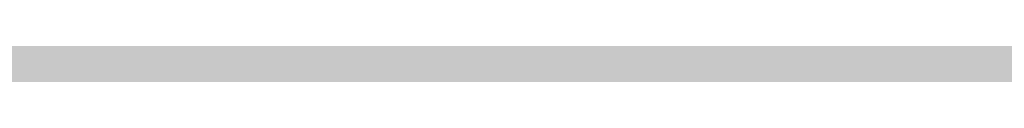
# Model space of a CAD drawing. Units: millimetres. Extents: x 0 to 2267, y 0 to 1823.
# Tile 55 of 256: x 1596.855 to 1600.369, y 1227.171 to 1227.246. Entities that reach past the tile are written whole.
import ezdxf

# ---------------------------------------------------------------- set-up
doc = ezdxf.new("R2010")
doc.units = ezdxf.units.MM
doc.header["$MEASUREMENT"] = 0
doc.layers.add('M-HATC', color=252, linetype='Continuous', lineweight=18)

msp = doc.modelspace()

# ---------------------------------------------------------------- hatches: boundary and pattern name
at = {"layer": 'M-HATC'}
h = msp.add_hatch(color=256, dxfattribs=at)
h.dxf.hatch_style = 1
h.paths.add_polyline_path([(2055.771, 1603.062), (1381.0868, 1603.062), (1381.0868, 1598.062), (2055.771, 1598.062)])
h.paths.add_polyline_path([(2055.771, 1598.062), (1381.0868, 1598.062), (1381.0868, 1593.062), (2055.771, 1593.062)])
h.paths.add_polyline_path([(2051.3074, 1536.7609), (1385.5504, 1536.7609), (1385.5504, 1526.7609), (1387.5504, 1526.7609), (1388.5366, 1525.0528), (1385.3319, 1521.2335), (1385.3319, 1521.2226), (2050.2542, 1522.7491), (2048.3212, 1525.0528), (2049.3074, 1526.7609), (2051.3074, 1526.7609)])
edge = h.paths.add_edge_path()
edge.add_arc((1847.5345, 1379.1492), 135, 222.603061, 222.890851, ccw=False)
edge.add_line((1748.1663, 1287.7656), (1683.0921, 1287.7656))
edge.add_arc((1583.7239, 1379.1492), 135, 317.109149, 317.396939, ccw=False)
edge.add_arc((1678.9686, 1290.6707), 5, 222.8909, 317.1091, ccw=False)
edge.add_arc((1774.2133, 1379.1492), 135, 222.603061, 222.890851, ccw=False)
edge.add_line((1674.8451, 1287.7656), (1609.7709, 1287.7656))
edge.add_arc((1510.4027, 1379.1492), 135, 317.109149, 317.396939, ccw=False)
edge.add_arc((1605.6474, 1290.6707), 5, 222.8909, 317.1091, ccw=False)
edge.add_arc((1700.8921, 1379.1492), 135, 222.603061, 222.890851, ccw=False)
edge.add_line((1601.5239, 1287.7656), (1536.4497, 1287.7656))
edge.add_arc((1437.0815, 1379.1492), 135, 317.109149, 317.396939, ccw=False)
edge.add_arc((1532.3262, 1290.6707), 5, 222.8909, 317.1091, ccw=False)
edge.add_arc((1627.5709, 1379.1492), 135, 222.603061, 222.890851, ccw=False)
edge.add_line((1528.2027, 1287.7656), (1505.9289, 1287.7656))
edge.add_spline(control_points=[(1505.9289, 1287.7656), (1504.2622, 1287.7656), (1504.2622, 1282.7656), (1505.9289, 1282.7656)], knot_values=[0, 0, 0, 0, 5, 5, 5, 5], degree=3, periodic=0)
edge.add_line((1505.9289, 1282.7656), (1930.9289, 1282.7656))
edge.add_spline(control_points=[(1930.9289, 1282.7656), (1932.5956, 1282.7656), (1932.5956, 1287.7656), (1930.9289, 1287.7656)], knot_values=[0, 0, 0, 0, 5, 5, 5, 5], degree=3, periodic=0)
edge.add_line((1930.9289, 1287.7656), (1903.0557, 1287.7656))
edge.add_arc((1803.6875, 1379.1492), 135, 317.109149, 317.396939, ccw=False)
edge.add_arc((1898.9322, 1290.6707), 5, 222.8909, 317.1091, ccw=False)
edge.add_arc((1994.1769, 1379.1492), 135, 222.603061, 222.890851, ccw=False)
edge.add_line((1894.8087, 1287.7656), (1829.7345, 1287.7656))
edge.add_arc((1730.3663, 1379.1492), 135, 317.109149, 317.396939, ccw=False)
edge.add_arc((1825.611, 1290.6707), 5, 222.8909, 317.1091, ccw=False)
edge.add_arc((1920.8557, 1379.1492), 135, 222.603061, 222.890851, ccw=False)
edge.add_line((1821.4875, 1287.7656), (1756.4133, 1287.7656))
edge.add_arc((1657.0451, 1379.1492), 135, 317.109149, 317.396939, ccw=False)
edge.add_arc((1752.2898, 1290.6707), 5, 222.8909, 317.1091, ccw=False)
edge = h.paths.add_edge_path()
edge.add_spline(control_points=[(1843.4289, 1227.2475), (1845.0956, 1227.2475), (1845.0956, 1232.2475), (1843.4289, 1232.2475)], knot_values=[0, 0, 0, 0, 5, 5, 5, 5], degree=3, periodic=0)
edge.add_line((1843.4289, 1232.2475), (1593.4289, 1232.2475))
edge.add_spline(control_points=[(1593.4289, 1232.2475), (1591.7622, 1232.2475), (1591.7622, 1227.2475), (1593.4289, 1227.2475)], knot_values=[0, 0, 0, 0, 5, 5, 5, 5], degree=3, periodic=0)
edge.add_line((1593.4289, 1227.2475), (1843.4289, 1227.2475))
h.paths.add_polyline_path([(1905.9289, 1127.4171), (1530.9289, 1127.4171, 0.414214), (1520.9289, 1117.4171), (1530.9289, 1117.4171), (1915.9289, 1117.4171, 0.414214)])
edge = h.paths.add_edge_path()
edge.add_arc((1397.0858, 1498.4078), 12.7299, 90.78215, 190.87871, ccw=False)
edge.add_line((1396.912, 1511.1365), (1428.0097, 1511.3488))
edge.add_line((1428.0097, 1511.3488), (1433.0097, 1511.3488))
edge.add_line((1433.0097, 1511.3488), (1434.439, 1511.3488))
edge.add_arc((1419.474, 1498.0804), 20, 41.561, 74.08211)
edge.add_line((1424.9592, 1517.3135), (1399.9351, 1517.2561))
edge.add_spline(control_points=[(1399.9307, 1517.2561), (1399.884, 1517.2131), (1399.8328, 1517.1689), (1399.7774, 1517.1236)], knot_values=[11.567499, 11.567499, 11.567499, 11.567499, 11.814249, 11.814249, 11.814249, 11.814249], degree=3, periodic=0)
edge.add_spline(control_points=[(1399.6328, 1517.0099), (1399.5831, 1516.9721), (1399.5307, 1516.9338), (1399.4759, 1516.8947)], knot_values=[11.167718, 11.167718, 11.167718, 11.167718, 11.365188, 11.365188, 11.365188, 11.365188], degree=3, periodic=0)
edge.add_spline(control_points=[(1399.3398, 1516.8001), (1399.1514, 1516.6719), (1398.9384, 1516.5377), (1398.704, 1516.3994)], knot_values=[10.376405, 10.376405, 10.376405, 10.376405, 11.00994, 11.00994, 11.00994, 11.00994], degree=3, periodic=0)
edge.add_spline(control_points=[(1398.6572, 1516.3719), (1398.5789, 1516.326), (1398.4983, 1516.2797), (1398.4155, 1516.2331)], knot_values=[10.125175, 10.125175, 10.125175, 10.125175, 10.334406, 10.334406, 10.334406, 10.334406], degree=3, periodic=0)
edge.add_spline(control_points=[(1398.2642, 1516.1487), (1398.196, 1516.1111), (1398.1263, 1516.0732), (1398.0555, 1516.0351)], knot_values=[9.832246, 9.832246, 9.832246, 9.832246, 9.999658, 9.999658, 9.999658, 9.999658], degree=3, periodic=0)
edge.add_spline(control_points=[(1397.9987, 1516.0048), (1397.7312, 1515.8621), (1397.446, 1515.7171), (1397.1466, 1515.5714)], knot_values=[9.161808, 9.161808, 9.161808, 9.161808, 9.787769, 9.787769, 9.787769, 9.787769], degree=3, periodic=0)
edge.add_spline(control_points=[(1397.1466, 1515.5714), (1396.8418, 1515.423), (1396.5222, 1515.274), (1396.1914, 1515.1262)], knot_values=[8.524455, 8.524455, 8.524455, 8.524455, 9.161808, 9.161808, 9.161808, 9.161808], degree=3, periodic=0)
edge.add_spline(control_points=[(1396.0777, 1515.0756), (1395.9854, 1515.0348), (1395.8922, 1514.994), (1395.7983, 1514.9534)], knot_values=[8.275193, 8.275193, 8.275193, 8.275193, 8.451726, 8.451726, 8.451726, 8.451726], degree=3, periodic=0)
edge.add_spline(control_points=[(1395.6018, 1514.8691), (1395.4997, 1514.8257), (1395.3968, 1514.7824), (1395.2932, 1514.7394)], knot_values=[7.962917, 7.962917, 7.962917, 7.962917, 8.152764, 8.152764, 8.152764, 8.152764], degree=3, periodic=0)
edge.add_spline(control_points=[(1395.2116, 1514.7057), (1394.8278, 1514.5475), (1394.4345, 1514.3929), (1394.0364, 1514.2442)], knot_values=[7.21254, 7.21254, 7.21254, 7.21254, 7.913148, 7.913148, 7.913148, 7.913148], degree=3, periodic=0)
edge.add_spline(control_points=[(1394.0364, 1514.2442), (1393.7076, 1514.1214), (1393.3754, 1514.0027), (1393.0427, 1513.8895)], knot_values=[6.633733, 6.633733, 6.633733, 6.633733, 7.21254, 7.21254, 7.21254, 7.21254], degree=3, periodic=0)
edge.add_spline(control_points=[(1392.8214, 1513.815), (1392.7198, 1513.7812), (1392.6181, 1513.7479), (1392.5166, 1513.7152)], knot_values=[6.328796, 6.328796, 6.328796, 6.328796, 6.505493, 6.505493, 6.505493, 6.505493], degree=3, periodic=0)
edge.add_spline(control_points=[(1392.5166, 1513.7152), (1392.3187, 1513.6515), (1392.1212, 1513.59), (1391.9244, 1513.531)], knot_values=[5.984605, 5.984605, 5.984605, 5.984605, 6.328796, 6.328796, 6.328796, 6.328796], degree=3, periodic=0)
edge.add_spline(control_points=[(1391.7915, 1513.4915), (1391.3122, 1513.3501), (1390.8384, 1513.2239), (1390.3784, 1513.1171)], knot_values=[5.066697, 5.066697, 5.066697, 5.066697, 5.907055, 5.907055, 5.907055, 5.907055], degree=3, periodic=0)
edge.add_spline(control_points=[(1390.3784, 1513.1171), (1390.1797, 1513.071), (1389.9836, 1513.0284), (1389.7907, 1512.9899)], knot_values=[4.70367, 4.70367, 4.70367, 4.70367, 5.066695, 5.066695, 5.066695, 5.066695], degree=3, periodic=0)
edge.add_spline(control_points=[(1389.422, 1512.9204), (1389.2459, 1512.8892), (1389.0729, 1512.8617), (1388.9036, 1512.8381)], knot_values=[4.130571, 4.130571, 4.130571, 4.130571, 4.469816, 4.469816, 4.469816, 4.469816], degree=3, periodic=0)
edge.add_spline(control_points=[(1388.9036, 1512.8381), (1388.591, 1512.7946), (1388.2911, 1512.7644), (1388.0071, 1512.7494)], knot_values=[3.504031, 3.504031, 3.504031, 3.504031, 4.130571, 4.130571, 4.130571, 4.130571], degree=3, periodic=0)
edge.add_spline(control_points=[(1387.9356, 1512.7459), (1387.8538, 1512.7423), (1387.7733, 1512.74), (1387.6944, 1512.739)], knot_values=[3.268866, 3.268866, 3.268866, 3.268866, 3.451164, 3.451164, 3.451164, 3.451164], degree=3, periodic=0)
edge.add_spline(control_points=[(1387.3351, 1512.7443), (1387.2076, 1512.7499), (1387.0847, 1512.7597), (1386.967, 1512.7739)], knot_values=[2.670686, 2.670686, 2.670686, 2.670686, 2.984, 2.984, 2.984, 2.984], degree=3, periodic=0)
edge.add_spline(control_points=[(1386.8327, 1512.7922), (1386.8209, 1512.7941), (1386.8092, 1512.7959), (1386.7975, 1512.7979)], knot_values=[2.516981, 2.516981, 2.516981, 2.516981, 2.549528, 2.549528, 2.549528, 2.549528], degree=3, periodic=0)
edge.add_spline(control_points=[(1386.4526, 1512.8735), (1386.4257, 1512.881), (1386.3993, 1512.889), (1386.3733, 1512.8972)], knot_values=[2.095869, 2.095869, 2.095869, 2.095869, 2.17941, 2.17941, 2.17941, 2.17941], degree=3, periodic=0)
edge.add_spline(control_points=[(1386.0691, 1513.0189), (1386.0634, 1513.0217), (1386.0577, 1513.0246), (1386.052, 1513.0275)], knot_values=[1.72453, 1.72453, 1.72453, 1.72453, 1.745933, 1.745933, 1.745933, 1.745933], degree=3, periodic=0)
edge.add_arc((1399.474, 1498.0804), 20, 131.82432, 180)
edge.add_arc((1630.3336, 1505.5484), 250.9708, 181.705176, 236.427975)
edge.add_arc((1605.3399, 1483.3044), 218.7822, 238.660829, 243.34961)
edge.add_arc((1647.0911, 1510.3592), 262.8986, 183.129836, 237.853442, ccw=False)
h.paths.add_polyline_path([(1406.5369, 1391.9644, 0.149382), (1491.5506, 1296.4418, -0.129517)], flags=17)
edge = h.paths.add_edge_path()
edge.add_arc((2037.3838, 1498.0804), 20, 0, 48.26587)
edge.add_spline(control_points=[(2050.6973, 1513.0052), (2050.6512, 1512.9847), (2050.6034, 1512.9655), (2050.5539, 1512.9477)], knot_values=[1.835652, 1.835652, 1.835652, 1.835652, 2.000781, 2.000781, 2.000781, 2.000781], degree=3, periodic=0)
edge.add_spline(control_points=[(2050.4616, 1512.9166), (2050.479, 1512.9221), (2050.4963, 1512.9277), (2050.5133, 1512.9335)], knot_values=[2.045477, 2.045477, 2.045477, 2.045477, 2.101389, 2.101389, 2.101389, 2.101389], degree=3, periodic=0)
edge.add_spline(control_points=[(2050.129, 1512.8342), (2050.1984, 1512.8473), (2050.2657, 1512.8623), (2050.3308, 1512.8792)], knot_values=[2.237629, 2.237629, 2.237629, 2.237629, 2.435841, 2.435841, 2.435841, 2.435841], degree=3, periodic=0)
edge.add_spline(control_points=[(2050.0946, 1512.8278), (2050.1061, 1512.8299), (2050.1176, 1512.832), (2050.129, 1512.8342)], knot_values=[2.435841, 2.435841, 2.435841, 2.435841, 2.468321, 2.468321, 2.468321, 2.468321], degree=3, periodic=0)
edge.add_spline(control_points=[(2049.7843, 1512.7851), (2049.8552, 1512.7922), (2049.9243, 1512.8008), (2049.9917, 1512.8109)], knot_values=[2.563852, 2.563852, 2.563852, 2.563852, 2.748541, 2.748541, 2.748541, 2.748541], degree=3, periodic=0)
edge.add_spline(control_points=[(2049.4052, 1512.7617), (2049.5364, 1512.7653), (2049.6629, 1512.773), (2049.7843, 1512.7851)], knot_values=[2.748541, 2.748541, 2.748541, 2.748541, 3.064882, 3.064882, 3.064882, 3.064882], degree=3, periodic=0)
edge.add_spline(control_points=[(2049.1698, 1512.7597), (2049.2336, 1512.7591), (2049.2965, 1512.7594), (2049.3584, 1512.7606)], knot_values=[3.102309, 3.102309, 3.102309, 3.102309, 3.2503, 3.2503, 3.2503, 3.2503], degree=3, periodic=0)
edge.add_spline(control_points=[(2048.8573, 1512.7691), (2048.9638, 1512.7638), (2049.068, 1512.7606), (2049.1698, 1512.7597)], knot_values=[3.2503, 3.2503, 3.2503, 3.2503, 3.486069, 3.486069, 3.486069, 3.486069], degree=3, periodic=0)
edge.add_spline(control_points=[(2048.6924, 1512.7789), (2048.3729, 1512.8009), (2048.0345, 1512.8411), (2047.6817, 1512.897)], knot_values=[3.606429, 3.606429, 3.606429, 3.606429, 4.2989, 4.2989, 4.2989, 4.2989], degree=3, periodic=0)
edge.add_spline(control_points=[(2047.6817, 1512.897), (2047.5458, 1512.9185), (2047.4077, 1512.9424), (2047.2678, 1512.9685)], knot_values=[4.2989, 4.2989, 4.2989, 4.2989, 4.565769, 4.565769, 4.565769, 4.565769], degree=3, periodic=0)
edge.add_spline(control_points=[(2047.2678, 1512.9685), (2047.1449, 1512.9914), (2047.0207, 1513.016), (2046.8951, 1513.0422)], knot_values=[4.565769, 4.565769, 4.565769, 4.565769, 4.799971, 4.799971, 4.799971, 4.799971], degree=3, periodic=0)
edge.add_spline(control_points=[(2046.8951, 1513.0422), (2046.5286, 1513.1188), (2046.1513, 1513.209), (2045.7676, 1513.3107)], knot_values=[4.799971, 4.799971, 4.799971, 4.799971, 5.483718, 5.483718, 5.483718, 5.483718], degree=3, periodic=0)
edge.add_spline(control_points=[(2045.7676, 1513.3107), (2045.3724, 1513.4154), (2044.9704, 1513.5322), (2044.5662, 1513.6588)], knot_values=[5.483718, 5.483718, 5.483718, 5.483718, 6.187866, 6.187866, 6.187866, 6.187866], degree=3, periodic=0)
edge.add_spline(control_points=[(2044.5662, 1513.6588), (2044.4149, 1513.7061), (2044.2633, 1513.7549), (2044.1116, 1513.8048)], knot_values=[6.187866, 6.187866, 6.187866, 6.187866, 6.451551, 6.451551, 6.451551, 6.451551], degree=3, periodic=0)
edge.add_spline(control_points=[(2044.1116, 1513.8048), (2043.9967, 1513.8427), (2043.8817, 1513.8813), (2043.7668, 1513.9205)], knot_values=[6.451551, 6.451551, 6.451551, 6.451551, 6.651434, 6.651434, 6.651434, 6.651434], degree=3, periodic=0)
edge.add_spline(control_points=[(2043.7668, 1513.9205), (2043.3716, 1514.0554), (2042.9774, 1514.1979), (2042.5886, 1514.3458)], knot_values=[6.651434, 6.651434, 6.651434, 6.651434, 7.338879, 7.338879, 7.338879, 7.338879], degree=3, periodic=0)
edge.add_spline(control_points=[(2042.5886, 1514.3458), (2042.1643, 1514.5071), (2041.7465, 1514.6749), (2041.3409, 1514.846)], knot_values=[7.338879, 7.338879, 7.338879, 7.338879, 8.089209, 8.089209, 8.089209, 8.089209], degree=3, periodic=0)
edge.add_spline(control_points=[(2041.3409, 1514.846), (2041.1028, 1514.9465), (2040.869, 1515.0481), (2040.6405, 1515.1502)], knot_values=[8.089209, 8.089209, 8.089209, 8.089209, 8.529587, 8.529587, 8.529587, 8.529587], degree=3, periodic=0)
edge.add_spline(control_points=[(2040.51, 1515.2089), (2040.0824, 1515.4022), (2039.6747, 1515.5971), (2039.295, 1515.7894)], knot_values=[8.613818, 8.613818, 8.613818, 8.613818, 9.44571, 9.44571, 9.44571, 9.44571], degree=3, periodic=0)
edge.add_spline(control_points=[(2039.295, 1515.7894), (2039.0618, 1515.9075), (2038.8391, 1516.0246), (2038.6288, 1516.1398)], knot_values=[9.44571, 9.44571, 9.44571, 9.44571, 9.956404, 9.956404, 9.956404, 9.956404], degree=3, periodic=0)
edge.add_spline(control_points=[(2038.6288, 1516.1398), (2038.5187, 1516.2001), (2038.4121, 1516.2598), (2038.309, 1516.3189)], knot_values=[9.956404, 9.956404, 9.956404, 9.956404, 10.223542, 10.223542, 10.223542, 10.223542], degree=3, periodic=0)
edge.add_spline(control_points=[(2038.309, 1516.3189), (2038.2138, 1516.3735), (2038.1216, 1516.4276), (2038.0328, 1516.481)], knot_values=[10.223542, 10.223542, 10.223542, 10.223542, 10.47051, 10.47051, 10.47051, 10.47051], degree=3, periodic=0)
edge.add_spline(control_points=[(2038.0328, 1516.481), (2037.7855, 1516.6296), (2037.5639, 1516.773), (2037.3722, 1516.909)], knot_values=[10.47051, 10.47051, 10.47051, 10.47051, 11.15767, 11.15767, 11.15767, 11.15767], degree=3, periodic=0)
edge.add_spline(control_points=[(2037.3722, 1516.909), (2037.2789, 1516.9752), (2037.1927, 1517.0396), (2037.1142, 1517.102)], knot_values=[11.15767, 11.15767, 11.15767, 11.15767, 11.49227, 11.49227, 11.49227, 11.49227], degree=3, periodic=0)
edge.add_spline(control_points=[(2036.8564, 1517.3259), (2036.9148, 1517.2692), (2036.9814, 1517.2103), (2037.0557, 1517.1492)], knot_values=[11.577341, 11.577341, 11.577341, 11.577341, 11.91035, 11.91035, 11.91035, 11.91035], degree=3, periodic=0)
edge.add_spline(control_points=[(2036.8074, 1517.3748), (2036.823, 1517.3587), (2036.8393, 1517.3424), (2036.8564, 1517.3259)], knot_values=[11.91035, 11.91035, 11.91035, 11.91035, 12.007402, 12.007402, 12.007402, 12.007402], degree=3, periodic=0)
edge.add_spline(control_points=[(2036.7017, 1517.494), (2036.7104, 1517.483), (2036.7196, 1517.4719), (2036.7291, 1517.4606)], knot_values=[12.184155, 12.184155, 12.184155, 12.184155, 12.255409, 12.255409, 12.255409, 12.255409], degree=3, periodic=0)
edge.add_spline(control_points=[(2036.6159, 1517.6205), (2036.62, 1517.613), (2036.6243, 1517.6055), (2036.6289, 1517.5979)], knot_values=[12.487913, 12.487913, 12.487913, 12.487913, 12.541035, 12.541035, 12.541035, 12.541035], degree=3, periodic=0)
edge.add_spline(control_points=[(2036.5635, 1517.786), (2036.5637, 1517.7794), (2036.5642, 1517.7726), (2036.565, 1517.7658)], knot_values=[12.911761, 12.911761, 12.911761, 12.911761, 12.968286, 12.968286, 12.968286, 12.968286], degree=3, periodic=0)
edge.add_spline(control_points=[(2036.6166, 1517.9304), (2036.6125, 1517.9259), (2036.6086, 1517.9212), (2036.6049, 1517.9165)], knot_values=[13.382527, 13.382527, 13.382527, 13.382527, 13.433791, 13.433791, 13.433791, 13.433791], degree=3, periodic=0)
edge.add_spline(control_points=[(2036.749, 1518.017), (2036.7361, 1518.0116), (2036.7239, 1518.006), (2036.7124, 1518.0002)], knot_values=[13.726299, 13.726299, 13.726299, 13.726299, 13.809928, 13.809928, 13.809928, 13.809928], degree=3, periodic=0)
edge.add_spline(control_points=[(2036.8604, 1518.0528), (2036.8386, 1518.0474), (2036.8181, 1518.0416), (2036.7988, 1518.0353)], knot_values=[13.910887, 13.910887, 13.910887, 13.910887, 14.02153, 14.02153, 14.02153, 14.02153], degree=3, periodic=0)
edge.add_line((2036.9639, 1518.0804), (2032.3838, 1518.0804))
edge.add_line((2032.3838, 1518.0804), (2027.3838, 1518.0804))
edge.add_line((2027.3838, 1518.0804), (2022.3838, 1518.0804))
edge.add_line((2022.3838, 1518.0804), (2017.3838, 1518.0804))
edge.add_arc((2017.3838, 1498.0804), 20, 90, 138.439)
edge.add_line((2002.4188, 1511.3488), (2003.8481, 1511.3488))
edge.add_line((2003.8481, 1511.3488), (2008.8481, 1511.3488))
edge.add_line((2008.8481, 1511.3488), (2039.772, 1511.1377))
edge.add_arc((2039.772, 1498.4078), 12.7299, -10.87871, 90, ccw=False)
edge.add_arc((1789.7668, 1510.3592), 262.8986, 302.146558, 356.870164, ccw=False)
edge.add_arc((1831.5179, 1483.3044), 218.7822, 296.65039, 301.339171)
edge.add_arc((1806.5242, 1505.5484), 250.9708, 303.572025, 358.294824)
h.paths.add_polyline_path([(2030.321, 1391.9644, -0.129517), (1945.3072, 1296.4418, 0.149382)], flags=17)
edge = h.paths.add_edge_path()
edge.add_spline(control_points=[(2037.2464, 1518.0821), (2037.2898, 1518.081), (2037.3355, 1518.0804), (2037.3838, 1518.0804)], knot_values=[0.000012, 0.000012, 0.000012, 0.000012, 0.144754, 0.144754, 0.144754, 0.144754], degree=3, periodic=0)
edge.add_line((2037.3357, 1518.0804), (2037.0096, 1518.0804))
edge.add_spline(control_points=[(2037.0096, 1518.0804), (2036.9822, 1518.0768), (2036.956, 1518.0727), (2036.9312, 1518.0681)], knot_values=[14.13465, 14.13465, 14.13465, 14.13465, 14.247197, 14.247197, 14.247197, 14.247197], degree=3, periodic=0)
edge.add_spline(control_points=[(2036.9312, 1518.0681), (2036.9276, 1518.0674), (2036.9241, 1518.0667), (2036.9205, 1518.0661)], knot_values=[14.118315, 14.118315, 14.118315, 14.118315, 14.13465, 14.13465, 14.13465, 14.13465], degree=3, periodic=0)
edge.add_spline(control_points=[(2036.9205, 1518.0661), (2036.9118, 1518.0644), (2036.9032, 1518.0626), (2036.8948, 1518.0608)], knot_values=[14.078086, 14.078086, 14.078086, 14.078086, 14.118315, 14.118315, 14.118315, 14.118315], degree=3, periodic=0)
edge.add_spline(control_points=[(2036.8948, 1518.0608), (2036.883, 1518.0583), (2036.8716, 1518.0556), (2036.8604, 1518.0528)], knot_values=[14.02153, 14.02153, 14.02153, 14.02153, 14.078086, 14.078086, 14.078086, 14.078086], degree=3, periodic=0)
edge.add_spline(control_points=[(2036.8604, 1518.0528), (2036.8386, 1518.0474), (2036.8181, 1518.0416), (2036.7988, 1518.0353)], knot_values=[13.910887, 13.910887, 13.910887, 13.910887, 14.02153, 14.02153, 14.02153, 14.02153], degree=3, periodic=0)
edge.add_spline(control_points=[(2036.7988, 1518.0353), (2036.7981, 1518.035), (2036.7974, 1518.0348), (2036.7967, 1518.0346)], knot_values=[13.906906, 13.906906, 13.906906, 13.906906, 13.910887, 13.910887, 13.910887, 13.910887], degree=3, periodic=0)
edge.add_spline(control_points=[(2036.7967, 1518.0346), (2036.7882, 1518.0318), (2036.7799, 1518.0289), (2036.7719, 1518.0259)], knot_values=[13.857826, 13.857826, 13.857826, 13.857826, 13.906906, 13.906906, 13.906906, 13.906906], degree=3, periodic=0)
edge.add_spline(control_points=[(2036.7719, 1518.0259), (2036.764, 1518.023), (2036.7564, 1518.02), (2036.749, 1518.017)], knot_values=[13.809928, 13.809928, 13.809928, 13.809928, 13.857826, 13.857826, 13.857826, 13.857826], degree=3, periodic=0)
edge.add_spline(control_points=[(2036.749, 1518.017), (2036.7361, 1518.0116), (2036.7239, 1518.006), (2036.7124, 1518.0002)], knot_values=[13.726299, 13.726299, 13.726299, 13.726299, 13.809928, 13.809928, 13.809928, 13.809928], degree=3, periodic=0)
edge.add_spline(control_points=[(2036.7124, 1518.0002), (2036.7121, 1518), (2036.7118, 1517.9999), (2036.7115, 1517.9997)], knot_values=[13.723993, 13.723993, 13.723993, 13.723993, 13.726299, 13.726299, 13.726299, 13.726299], degree=3, periodic=0)
edge.add_spline(control_points=[(2036.7115, 1517.9997), (2036.7063, 1517.9971), (2036.7013, 1517.9944), (2036.6965, 1517.9917)], knot_values=[13.686536, 13.686536, 13.686536, 13.686536, 13.723993, 13.723993, 13.723993, 13.723993], degree=3, periodic=0)
edge.add_spline(control_points=[(2036.6965, 1517.9917), (2036.6919, 1517.9891), (2036.6874, 1517.9865), (2036.6831, 1517.9839)], knot_values=[13.651251, 13.651251, 13.651251, 13.651251, 13.686536, 13.686536, 13.686536, 13.686536], degree=3, periodic=0)
edge.add_spline(control_points=[(2036.6831, 1517.9839), (2036.6764, 1517.9798), (2036.67, 1517.9757), (2036.6639, 1517.9714)], knot_values=[13.596804, 13.596804, 13.596804, 13.596804, 13.651251, 13.651251, 13.651251, 13.651251], degree=3, periodic=0)
edge.add_spline(control_points=[(2036.6639, 1517.9714), (2036.6636, 1517.9712), (2036.6633, 1517.9709), (2036.6629, 1517.9707)], knot_values=[13.593956, 13.593956, 13.593956, 13.593956, 13.596804, 13.596804, 13.596804, 13.596804], degree=3, periodic=0)
edge.add_spline(control_points=[(2036.6629, 1517.9707), (2036.6603, 1517.9689), (2036.6577, 1517.967), (2036.6552, 1517.9651)], knot_values=[13.570322, 13.570322, 13.570322, 13.570322, 13.593956, 13.593956, 13.593956, 13.593956], degree=3, periodic=0)
edge.add_spline(control_points=[(2036.6552, 1517.9651), (2036.6525, 1517.9631), (2036.6499, 1517.9611), (2036.6474, 1517.9591)], knot_values=[13.545477, 13.545477, 13.545477, 13.545477, 13.570322, 13.570322, 13.570322, 13.570322], degree=3, periodic=0)
edge.add_spline(control_points=[(2036.6474, 1517.9591), (2036.6472, 1517.9589), (2036.6471, 1517.9588), (2036.6469, 1517.9587)], knot_values=[13.543931, 13.543931, 13.543931, 13.543931, 13.545477, 13.545477, 13.545477, 13.545477], degree=3, periodic=0)
edge.add_spline(control_points=[(2036.6469, 1517.9587), (2036.6412, 1517.9541), (2036.6358, 1517.9494), (2036.6307, 1517.9447)], knot_values=[13.488237, 13.488237, 13.488237, 13.488237, 13.543931, 13.543931, 13.543931, 13.543931], degree=3, periodic=0)
edge.add_spline(control_points=[(2036.6307, 1517.9447), (2036.6282, 1517.9423), (2036.6257, 1517.9399), (2036.6233, 1517.9374)], knot_values=[13.460307, 13.460307, 13.460307, 13.460307, 13.488237, 13.488237, 13.488237, 13.488237], degree=3, periodic=0)
edge.add_spline(control_points=[(2036.6233, 1517.9374), (2036.6215, 1517.9356), (2036.6198, 1517.9338), (2036.6181, 1517.932)], knot_values=[13.439712, 13.439712, 13.439712, 13.439712, 13.460307, 13.460307, 13.460307, 13.460307], degree=3, periodic=0)
edge.add_spline(control_points=[(2036.6181, 1517.932), (2036.6176, 1517.9315), (2036.6171, 1517.9309), (2036.6166, 1517.9304)], knot_values=[13.433791, 13.433791, 13.433791, 13.433791, 13.439712, 13.439712, 13.439712, 13.439712], degree=3, periodic=0)
edge.add_spline(control_points=[(2036.6166, 1517.9304), (2036.6125, 1517.9259), (2036.6086, 1517.9212), (2036.6049, 1517.9165)], knot_values=[13.382527, 13.382527, 13.382527, 13.382527, 13.433791, 13.433791, 13.433791, 13.433791], degree=3, periodic=0)
edge.add_spline(control_points=[(2036.6049, 1517.9165), (2036.6026, 1517.9135), (2036.6004, 1517.9104), (2036.5982, 1517.9074)], knot_values=[13.350017, 13.350017, 13.350017, 13.350017, 13.382527, 13.382527, 13.382527, 13.382527], degree=3, periodic=0)
edge.add_spline(control_points=[(2036.5982, 1517.9074), (2036.5972, 1517.9059), (2036.5962, 1517.9043), (2036.5952, 1517.9028)], knot_values=[13.333922, 13.333922, 13.333922, 13.333922, 13.350017, 13.350017, 13.350017, 13.350017], degree=3, periodic=0)
edge.add_spline(control_points=[(2036.5952, 1517.9028), (2036.5945, 1517.9018), (2036.5939, 1517.9009), (2036.5933, 1517.8999)], knot_values=[13.323828, 13.323828, 13.323828, 13.323828, 13.333922, 13.333922, 13.333922, 13.333922], degree=3, periodic=0)
edge.add_spline(control_points=[(2036.5933, 1517.8999), (2036.5905, 1517.8955), (2036.5879, 1517.8909), (2036.5855, 1517.8864)], knot_values=[13.277545, 13.277545, 13.277545, 13.277545, 13.323828, 13.323828, 13.323828, 13.323828], degree=3, periodic=0)
edge.add_spline(control_points=[(2036.5855, 1517.8864), (2036.5836, 1517.8827), (2036.5817, 1517.8789), (2036.5801, 1517.8751)], knot_values=[13.240119, 13.240119, 13.240119, 13.240119, 13.277545, 13.277545, 13.277545, 13.277545], degree=3, periodic=0)
edge.add_spline(control_points=[(2036.5801, 1517.8751), (2036.5795, 1517.8739), (2036.579, 1517.8727), (2036.5785, 1517.8715)], knot_values=[13.228211, 13.228211, 13.228211, 13.228211, 13.240119, 13.240119, 13.240119, 13.240119], degree=3, periodic=0)
edge.add_spline(control_points=[(2036.5785, 1517.8715), (2036.578, 1517.8702), (2036.5774, 1517.869), (2036.5769, 1517.8677)], knot_values=[13.215717, 13.215717, 13.215717, 13.215717, 13.228211, 13.228211, 13.228211, 13.228211], degree=3, periodic=0)
edge.add_spline(control_points=[(2036.5769, 1517.8677), (2036.5755, 1517.864), (2036.5741, 1517.8603), (2036.5729, 1517.8565)], knot_values=[13.179847, 13.179847, 13.179847, 13.179847, 13.215717, 13.215717, 13.215717, 13.215717], degree=3, periodic=0)
edge.add_spline(control_points=[(2036.5729, 1517.8565), (2036.5713, 1517.8515), (2036.5699, 1517.8464), (2036.5687, 1517.8413)], knot_values=[13.132017, 13.132017, 13.132017, 13.132017, 13.179847, 13.179847, 13.179847, 13.179847], degree=3, periodic=0)
edge.add_spline(control_points=[(2036.5687, 1517.8413), (2036.5684, 1517.8402), (2036.5682, 1517.8392), (2036.568, 1517.8382)], knot_values=[13.122482, 13.122482, 13.122482, 13.122482, 13.132017, 13.132017, 13.132017, 13.132017], degree=3, periodic=0)
edge.add_spline(control_points=[(2036.568, 1517.8382), (2036.5676, 1517.8363), (2036.5672, 1517.8345), (2036.5669, 1517.8327)], knot_values=[13.105592, 13.105592, 13.105592, 13.105592, 13.122482, 13.122482, 13.122482, 13.122482], degree=3, periodic=0)
edge.add_spline(control_points=[(2036.5669, 1517.8327), (2036.5662, 1517.8292), (2036.5657, 1517.8257), (2036.5652, 1517.8222)], knot_values=[13.074063, 13.074063, 13.074063, 13.074063, 13.105592, 13.105592, 13.105592, 13.105592], degree=3, periodic=0)
edge.add_spline(control_points=[(2036.5652, 1517.8222), (2036.5652, 1517.8222), (2036.5652, 1517.8222), (2036.5652, 1517.8222)], knot_values=[13.074043, 13.074043, 13.074043, 13.074043, 13.074063, 13.074063, 13.074063, 13.074063], degree=3, periodic=0)
edge.add_spline(control_points=[(2036.5652, 1517.8222), (2036.5644, 1517.8164), (2036.5639, 1517.8106), (2036.5636, 1517.8046)], knot_values=[13.021884, 13.021884, 13.021884, 13.021884, 13.074043, 13.074043, 13.074043, 13.074043], degree=3, periodic=0)
edge.add_spline(control_points=[(2036.5636, 1517.8046), (2036.5636, 1517.804), (2036.5636, 1517.8034), (2036.5635, 1517.8028)], knot_values=[13.01674, 13.01674, 13.01674, 13.01674, 13.021884, 13.021884, 13.021884, 13.021884], degree=3, periodic=0)
edge.add_spline(control_points=[(2036.5635, 1517.8028), (2036.5634, 1517.8005), (2036.5634, 1517.7982), (2036.5634, 1517.7958)], knot_values=[12.996438, 12.996438, 12.996438, 12.996438, 13.01674, 13.01674, 13.01674, 13.01674], degree=3, periodic=0)
edge.add_spline(control_points=[(2036.5634, 1517.7958), (2036.5633, 1517.7926), (2036.5634, 1517.7893), (2036.5635, 1517.786)], knot_values=[12.968286, 12.968286, 12.968286, 12.968286, 12.996438, 12.996438, 12.996438, 12.996438], degree=3, periodic=0)
edge.add_spline(control_points=[(2036.5635, 1517.786), (2036.5637, 1517.7794), (2036.5642, 1517.7726), (2036.565, 1517.7658)], knot_values=[12.911761, 12.911761, 12.911761, 12.911761, 12.968286, 12.968286, 12.968286, 12.968286], degree=3, periodic=0)
edge.add_spline(control_points=[(2036.565, 1517.7658), (2036.565, 1517.7657), (2036.565, 1517.7656), (2036.565, 1517.7656)], knot_values=[12.911017, 12.911017, 12.911017, 12.911017, 12.911761, 12.911761, 12.911761, 12.911761], degree=3, periodic=0)
edge.add_spline(control_points=[(2036.565, 1517.7656), (2036.5654, 1517.7625), (2036.5658, 1517.7593), (2036.5663, 1517.7562)], knot_values=[12.88528, 12.88528, 12.88528, 12.88528, 12.911017, 12.911017, 12.911017, 12.911017], degree=3, periodic=0)
edge.add_spline(control_points=[(2036.5663, 1517.7562), (2036.5667, 1517.7534), (2036.5672, 1517.7506), (2036.5677, 1517.7478)], knot_values=[12.862519, 12.862519, 12.862519, 12.862519, 12.88528, 12.88528, 12.88528, 12.88528], degree=3, periodic=0)
edge.add_spline(control_points=[(2036.5677, 1517.7478), (2036.5678, 1517.7474), (2036.5679, 1517.7469), (2036.568, 1517.7465)], knot_values=[12.858885, 12.858885, 12.858885, 12.858885, 12.862519, 12.862519, 12.862519, 12.862519], degree=3, periodic=0)
edge.add_spline(control_points=[(2036.568, 1517.7465), (2036.5692, 1517.7399), (2036.5707, 1517.7332), (2036.5724, 1517.7264)], knot_values=[12.8053, 12.8053, 12.8053, 12.8053, 12.858885, 12.858885, 12.858885, 12.858885], degree=3, periodic=0)
edge.add_spline(control_points=[(2036.5724, 1517.7264), (2036.5734, 1517.7226), (2036.5745, 1517.7187), (2036.5756, 1517.7149)], knot_values=[12.775176, 12.775176, 12.775176, 12.775176, 12.8053, 12.8053, 12.8053, 12.8053], degree=3, periodic=0)
edge.add_spline(control_points=[(2036.5756, 1517.7149), (2036.5763, 1517.7125), (2036.577, 1517.7102), (2036.5778, 1517.7078)], knot_values=[12.756759, 12.756759, 12.756759, 12.756759, 12.775176, 12.775176, 12.775176, 12.775176], degree=3, periodic=0)
edge.add_spline(control_points=[(2036.5778, 1517.7078), (2036.5781, 1517.7067), (2036.5784, 1517.7057), (2036.5787, 1517.7047)], knot_values=[12.748742, 12.748742, 12.748742, 12.748742, 12.756759, 12.756759, 12.756759, 12.756759], degree=3, periodic=0)
edge.add_spline(control_points=[(2036.5787, 1517.7047), (2036.5808, 1517.6983), (2036.5831, 1517.6919), (2036.5856, 1517.6854)], knot_values=[12.69959, 12.69959, 12.69959, 12.69959, 12.748742, 12.748742, 12.748742, 12.748742], degree=3, periodic=0)
edge.add_spline(control_points=[(2036.5856, 1517.6854), (2036.5876, 1517.68), (2036.5898, 1517.6746), (2036.5921, 1517.6692)], knot_values=[12.659038, 12.659038, 12.659038, 12.659038, 12.69959, 12.69959, 12.69959, 12.69959], degree=3, periodic=0)
edge.add_spline(control_points=[(2036.5921, 1517.6692), (2036.594, 1517.6648), (2036.5959, 1517.6605), (2036.5979, 1517.6561)], knot_values=[12.626806, 12.626806, 12.626806, 12.626806, 12.659038, 12.659038, 12.659038, 12.659038], degree=3, periodic=0)
edge.add_spline(control_points=[(2036.5979, 1517.6561), (2036.5984, 1517.6551), (2036.5989, 1517.6541), (2036.5993, 1517.6531)], knot_values=[12.619394, 12.619394, 12.619394, 12.619394, 12.626806, 12.626806, 12.626806, 12.626806], degree=3, periodic=0)
edge.add_spline(control_points=[(2036.5993, 1517.6531), (2036.6043, 1517.6424), (2036.6099, 1517.6315), (2036.6159, 1517.6205)], knot_values=[12.541039, 12.541039, 12.541039, 12.541039, 12.619394, 12.619394, 12.619394, 12.619394], degree=3, periodic=0)
edge.add_spline(control_points=[(2036.6159, 1517.6205), (2036.6159, 1517.6205), (2036.6159, 1517.6205), (2036.6159, 1517.6205)], knot_values=[12.541035, 12.541035, 12.541035, 12.541035, 12.541039, 12.541039, 12.541039, 12.541039], degree=3, periodic=0)
edge.add_spline(control_points=[(2036.6159, 1517.6205), (2036.62, 1517.613), (2036.6243, 1517.6055), (2036.6289, 1517.5979)], knot_values=[12.487913, 12.487913, 12.487913, 12.487913, 12.541035, 12.541035, 12.541035, 12.541035], degree=3, periodic=0)
edge.add_spline(control_points=[(2036.6289, 1517.5979), (2036.6326, 1517.5916), (2036.6365, 1517.5853), (2036.6406, 1517.5789)], knot_values=[12.443982, 12.443982, 12.443982, 12.443982, 12.487913, 12.487913, 12.487913, 12.487913], degree=3, periodic=0)
edge.add_spline(control_points=[(2036.6406, 1517.5789), (2036.6414, 1517.5776), (2036.6423, 1517.5763), (2036.6431, 1517.5749)], knot_values=[12.434996, 12.434996, 12.434996, 12.434996, 12.443982, 12.443982, 12.443982, 12.443982], degree=3, periodic=0)
edge.add_spline(control_points=[(2036.6431, 1517.5749), (2036.6531, 1517.5596), (2036.6639, 1517.5439), (2036.6756, 1517.528)], knot_values=[12.329647, 12.329647, 12.329647, 12.329647, 12.434996, 12.434996, 12.434996, 12.434996], degree=3, periodic=0)
edge.add_spline(control_points=[(2036.6756, 1517.528), (2036.6839, 1517.5168), (2036.6925, 1517.5055), (2036.7017, 1517.494)], knot_values=[12.255409, 12.255409, 12.255409, 12.255409, 12.329647, 12.329647, 12.329647, 12.329647], degree=3, periodic=0)
edge.add_spline(control_points=[(2036.7017, 1517.494), (2036.7104, 1517.483), (2036.7196, 1517.4719), (2036.7291, 1517.4606)], knot_values=[12.184155, 12.184155, 12.184155, 12.184155, 12.255409, 12.255409, 12.255409, 12.255409], degree=3, periodic=0)
edge.add_spline(control_points=[(2036.7291, 1517.4606), (2036.7436, 1517.4435), (2036.759, 1517.4262), (2036.7753, 1517.4085)], knot_values=[12.075961, 12.075961, 12.075961, 12.075961, 12.184155, 12.184155, 12.184155, 12.184155], degree=3, periodic=0)
edge.add_spline(control_points=[(2036.7753, 1517.4085), (2036.7763, 1517.4075), (2036.7773, 1517.4064), (2036.7783, 1517.4054)], knot_values=[12.069502, 12.069502, 12.069502, 12.069502, 12.075961, 12.075961, 12.075961, 12.075961], degree=3, periodic=0)
edge.add_spline(control_points=[(2036.7783, 1517.4054), (2036.7877, 1517.3953), (2036.7974, 1517.385), (2036.8074, 1517.3748)], knot_values=[12.007402, 12.007402, 12.007402, 12.007402, 12.069502, 12.069502, 12.069502, 12.069502], degree=3, periodic=0)
edge.add_spline(control_points=[(2036.8074, 1517.3748), (2036.823, 1517.3587), (2036.8393, 1517.3424), (2036.8564, 1517.3259)], knot_values=[11.91035, 11.91035, 11.91035, 11.91035, 12.007402, 12.007402, 12.007402, 12.007402], degree=3, periodic=0)
edge.add_spline(control_points=[(2036.8564, 1517.3259), (2036.9148, 1517.2692), (2036.9814, 1517.2103), (2037.0557, 1517.1492)], knot_values=[11.577341, 11.577341, 11.577341, 11.577341, 11.91035, 11.91035, 11.91035, 11.91035], degree=3, periodic=0)
edge.add_spline(control_points=[(2037.0557, 1517.1492), (2037.0747, 1517.1336), (2037.0942, 1517.1179), (2037.1142, 1517.102)], knot_values=[11.49227, 11.49227, 11.49227, 11.49227, 11.577341, 11.577341, 11.577341, 11.577341], degree=3, periodic=0)
edge.add_spline(control_points=[(2037.1142, 1517.102), (2037.1927, 1517.0396), (2037.2789, 1516.9752), (2037.3722, 1516.909)], knot_values=[11.15767, 11.15767, 11.15767, 11.15767, 11.49227, 11.49227, 11.49227, 11.49227], degree=3, periodic=0)
edge.add_spline(control_points=[(2037.3722, 1516.909), (2037.5639, 1516.773), (2037.7855, 1516.6296), (2038.0328, 1516.481)], knot_values=[10.47051, 10.47051, 10.47051, 10.47051, 11.15767, 11.15767, 11.15767, 11.15767], degree=3, periodic=0)
edge.add_spline(control_points=[(2038.0328, 1516.481), (2038.1216, 1516.4276), (2038.2138, 1516.3735), (2038.309, 1516.3189)], knot_values=[10.223542, 10.223542, 10.223542, 10.223542, 10.47051, 10.47051, 10.47051, 10.47051], degree=3, periodic=0)
edge.add_spline(control_points=[(2038.309, 1516.3189), (2038.4121, 1516.2598), (2038.5187, 1516.2001), (2038.6288, 1516.1398)], knot_values=[9.956404, 9.956404, 9.956404, 9.956404, 10.223542, 10.223542, 10.223542, 10.223542], degree=3, periodic=0)
edge.add_spline(control_points=[(2038.6288, 1516.1398), (2038.8391, 1516.0246), (2039.0618, 1515.9075), (2039.295, 1515.7894)], knot_values=[9.44571, 9.44571, 9.44571, 9.44571, 9.956404, 9.956404, 9.956404, 9.956404], degree=3, periodic=0)
edge.add_spline(control_points=[(2039.295, 1515.7894), (2039.6747, 1515.5971), (2040.0824, 1515.4022), (2040.51, 1515.2089)], knot_values=[8.613818, 8.613818, 8.613818, 8.613818, 9.44571, 9.44571, 9.44571, 9.44571], degree=3, periodic=0)
edge.add_spline(control_points=[(2040.51, 1515.2089), (2040.5533, 1515.1893), (2040.5968, 1515.1697), (2040.6405, 1515.1502)], knot_values=[8.529587, 8.529587, 8.529587, 8.529587, 8.613818, 8.613818, 8.613818, 8.613818], degree=3, periodic=0)
edge.add_spline(control_points=[(2040.6405, 1515.1502), (2040.869, 1515.0481), (2041.1028, 1514.9465), (2041.3409, 1514.846)], knot_values=[8.089209, 8.089209, 8.089209, 8.089209, 8.529587, 8.529587, 8.529587, 8.529587], degree=3, periodic=0)
edge.add_spline(control_points=[(2041.3409, 1514.846), (2041.7465, 1514.6749), (2042.1643, 1514.5071), (2042.5886, 1514.3458)], knot_values=[7.338879, 7.338879, 7.338879, 7.338879, 8.089209, 8.089209, 8.089209, 8.089209], degree=3, periodic=0)
edge.add_spline(control_points=[(2042.5886, 1514.3458), (2042.9774, 1514.1979), (2043.3716, 1514.0554), (2043.7668, 1513.9205)], knot_values=[6.651434, 6.651434, 6.651434, 6.651434, 7.338879, 7.338879, 7.338879, 7.338879], degree=3, periodic=0)
edge.add_spline(control_points=[(2043.7668, 1513.9205), (2043.8817, 1513.8813), (2043.9967, 1513.8427), (2044.1116, 1513.8048)], knot_values=[6.451551, 6.451551, 6.451551, 6.451551, 6.651434, 6.651434, 6.651434, 6.651434], degree=3, periodic=0)
edge.add_spline(control_points=[(2044.1116, 1513.8048), (2044.2633, 1513.7549), (2044.4149, 1513.7061), (2044.5662, 1513.6588)], knot_values=[6.187866, 6.187866, 6.187866, 6.187866, 6.451551, 6.451551, 6.451551, 6.451551], degree=3, periodic=0)
edge.add_spline(control_points=[(2044.5662, 1513.6588), (2044.9704, 1513.5322), (2045.3724, 1513.4154), (2045.7676, 1513.3107)], knot_values=[5.483718, 5.483718, 5.483718, 5.483718, 6.187866, 6.187866, 6.187866, 6.187866], degree=3, periodic=0)
edge.add_spline(control_points=[(2045.7676, 1513.3107), (2046.1513, 1513.209), (2046.5286, 1513.1188), (2046.8951, 1513.0422)], knot_values=[4.799971, 4.799971, 4.799971, 4.799971, 5.483718, 5.483718, 5.483718, 5.483718], degree=3, periodic=0)
edge.add_spline(control_points=[(2046.8951, 1513.0422), (2047.0207, 1513.016), (2047.1449, 1512.9914), (2047.2678, 1512.9685)], knot_values=[4.565769, 4.565769, 4.565769, 4.565769, 4.799971, 4.799971, 4.799971, 4.799971], degree=3, periodic=0)
edge.add_spline(control_points=[(2047.2678, 1512.9685), (2047.4077, 1512.9424), (2047.5458, 1512.9185), (2047.6817, 1512.897)], knot_values=[4.2989, 4.2989, 4.2989, 4.2989, 4.565769, 4.565769, 4.565769, 4.565769], degree=3, periodic=0)
edge.add_spline(control_points=[(2047.6817, 1512.897), (2048.0345, 1512.8411), (2048.3729, 1512.8009), (2048.6924, 1512.7789)], knot_values=[3.606429, 3.606429, 3.606429, 3.606429, 4.2989, 4.2989, 4.2989, 4.2989], degree=3, periodic=0)
edge.add_spline(control_points=[(2048.6924, 1512.7789), (2048.7479, 1512.7751), (2048.8029, 1512.7718), (2048.8573, 1512.7691)], knot_values=[3.486069, 3.486069, 3.486069, 3.486069, 3.606429, 3.606429, 3.606429, 3.606429], degree=3, periodic=0)
edge.add_spline(control_points=[(2048.8573, 1512.7691), (2048.9638, 1512.7638), (2049.068, 1512.7606), (2049.1698, 1512.7597)], knot_values=[3.2503, 3.2503, 3.2503, 3.2503, 3.486069, 3.486069, 3.486069, 3.486069], degree=3, periodic=0)
edge.add_spline(control_points=[(2049.1698, 1512.7597), (2049.2336, 1512.7591), (2049.2965, 1512.7594), (2049.3584, 1512.7606)], knot_values=[3.102309, 3.102309, 3.102309, 3.102309, 3.2503, 3.2503, 3.2503, 3.2503], degree=3, periodic=0)
edge.add_spline(control_points=[(2049.3584, 1512.7606), (2049.3741, 1512.7609), (2049.3897, 1512.7613), (2049.4052, 1512.7617)], knot_values=[3.064882, 3.064882, 3.064882, 3.064882, 3.102309, 3.102309, 3.102309, 3.102309], degree=3, periodic=0)
edge.add_spline(control_points=[(2049.4052, 1512.7617), (2049.5364, 1512.7653), (2049.6629, 1512.773), (2049.7843, 1512.7851)], knot_values=[2.748541, 2.748541, 2.748541, 2.748541, 3.064882, 3.064882, 3.064882, 3.064882], degree=3, periodic=0)
edge.add_spline(control_points=[(2049.7843, 1512.7851), (2049.8552, 1512.7922), (2049.9243, 1512.8008), (2049.9917, 1512.8109)], knot_values=[2.563852, 2.563852, 2.563852, 2.563852, 2.748541, 2.748541, 2.748541, 2.748541], degree=3, periodic=0)
edge.add_spline(control_points=[(2049.9917, 1512.8109), (2050.0265, 1512.8161), (2050.0608, 1512.8218), (2050.0946, 1512.8278)], knot_values=[2.468321, 2.468321, 2.468321, 2.468321, 2.563852, 2.563852, 2.563852, 2.563852], degree=3, periodic=0)
edge.add_spline(control_points=[(2050.0946, 1512.8278), (2050.1061, 1512.8299), (2050.1176, 1512.832), (2050.129, 1512.8342)], knot_values=[2.435841, 2.435841, 2.435841, 2.435841, 2.468321, 2.468321, 2.468321, 2.468321], degree=3, periodic=0)
edge.add_spline(control_points=[(2050.129, 1512.8342), (2050.1984, 1512.8473), (2050.2657, 1512.8623), (2050.3308, 1512.8792)], knot_values=[2.237629, 2.237629, 2.237629, 2.237629, 2.435841, 2.435841, 2.435841, 2.435841], degree=3, periodic=0)
edge.add_spline(control_points=[(2050.3308, 1512.8792), (2050.3754, 1512.8908), (2050.4191, 1512.9032), (2050.4616, 1512.9166)], knot_values=[2.101389, 2.101389, 2.101389, 2.101389, 2.237629, 2.237629, 2.237629, 2.237629], degree=3, periodic=0)
edge.add_spline(control_points=[(2050.4616, 1512.9166), (2050.479, 1512.9221), (2050.4963, 1512.9277), (2050.5133, 1512.9335)], knot_values=[2.045477, 2.045477, 2.045477, 2.045477, 2.101389, 2.101389, 2.101389, 2.101389], degree=3, periodic=0)
edge.add_spline(control_points=[(2050.5133, 1512.9335), (2050.527, 1512.9382), (2050.5405, 1512.9429), (2050.5539, 1512.9477)], knot_values=[2.000781, 2.000781, 2.000781, 2.000781, 2.045477, 2.045477, 2.045477, 2.045477], degree=3, periodic=0)
edge.add_spline(control_points=[(2050.5539, 1512.9477), (2050.6034, 1512.9655), (2050.6512, 1512.9847), (2050.6973, 1513.0052)], knot_values=[1.835652, 1.835652, 1.835652, 1.835652, 2.000781, 2.000781, 2.000781, 2.000781], degree=3, periodic=0)
edge.add_arc((2037.3838, 1498.0804), 20, 48.26587, 90.12993)
edge = h.paths.add_edge_path(flags=16)
edge.add_spline(control_points=[(1386.1389, 1512.9859), (1388.92, 1511.7395), (1398.0387, 1515.5187), (1399.9307, 1517.2561)], knot_values=[1.831046, 1.831046, 1.831046, 1.831046, 11.814249, 11.814249, 11.814249, 11.814249], degree=3, periodic=0)
edge.add_line((1399.9307, 1517.2561), (1393.7435, 1517.2419))
edge.add_arc((1399.474, 1498.0804), 20, 106.6501, 131.8173)
h = msp.add_hatch(color=256, dxfattribs=at)
h.dxf.hatch_style = 1
h.paths.add_polyline_path([(2042.8886, 1580.1796), (2055.771, 1593.062), (1381.0868, 1593.062), (1393.9692, 1580.1796), (1374.086, 1560.2964), (2062.7718, 1560.2964)])
h.paths.add_polyline_path([(1843.4289, 1201.3297), (1843.4289, 1227.2475), (1593.4289, 1227.2475), (1593.4289, 1201.3297, -0.228274), (1574.5989, 1162.2346), (1530.9289, 1127.4171), (1905.9289, 1127.4171), (1862.2589, 1162.2346, -0.228274)])

doc.saveas('drawing.dxf')
